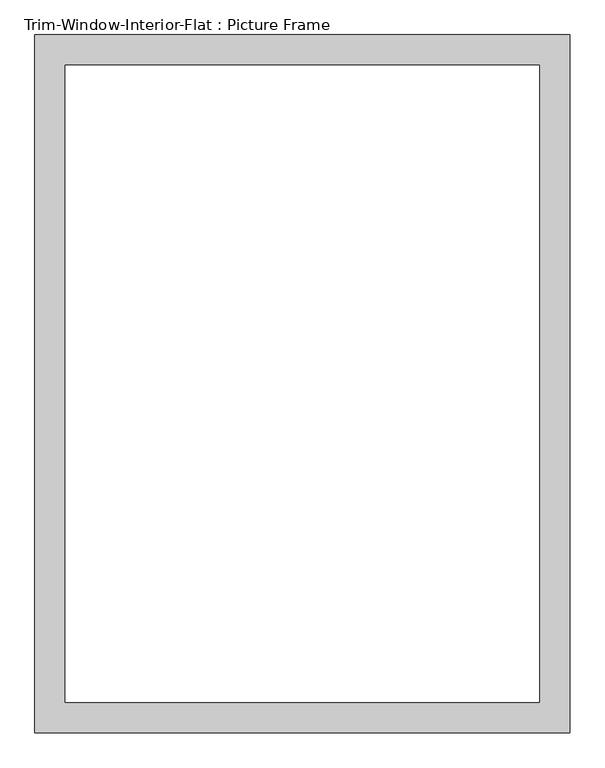
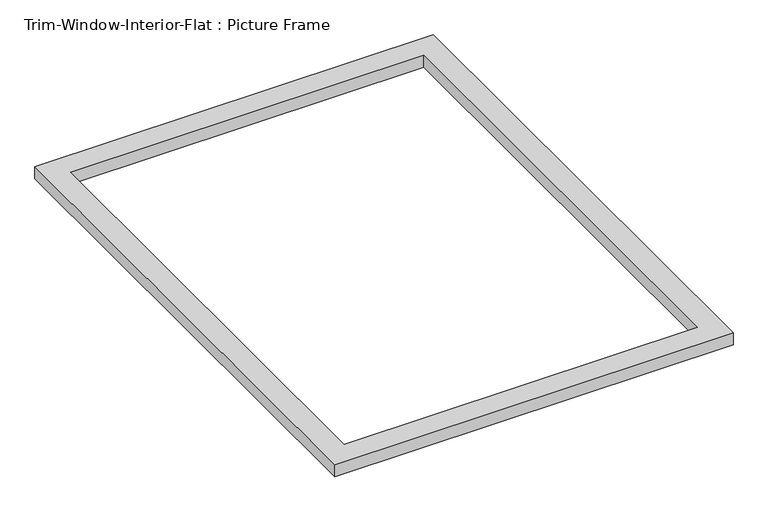
"""IFC4 building model written with IfcOpenShell, lengths in millimetres: proxy geometry, Trim-Window-Interior-Flat : Picture Frame."""

from ifc_helpers import new_model, si_unit, origin, origin_with_axes, place, context, project, spatial, polyline, outline, extrude, source, transform, mapped, element, save


def trim_window_interior_flat_picture_frame_c1dcbb6d(model_context):
    return source(origin(), model_context, "Body", "SweptSolid", [
        extrude(outline(polyline([(501.65, -44.45), (-501.65, -44.45), (-501.65, 1263.65), (501.65, 1263.65), (501.65, -44.45)]), holes=[polyline([(444.5, 12.7), (444.5, 1206.5), (-444.5, 1206.5), (-444.5, 12.7), (444.5, 12.7)])]), origin_with_axes(), (0.0, 0.0, 1.0), 31.75),
    ])


if __name__ == "__main__":
    model = new_model("IFC4")
    model_context = context("Model", 3, world=origin())
    ifc_project = project(units=[si_unit("LENGTHUNIT", "METRE", prefix="MILLI")], contexts=[model_context])
    site = spatial("IfcSite", under=ifc_project)
    building = spatial("IfcBuilding", under=site)
    placement = place(None, origin())
    trim_window_interior_flat_picture_frame_shape = trim_window_interior_flat_picture_frame_c1dcbb6d(model_context)
    element("IfcBuildingElementProxy", 1, Name="Trim-Window-Interior-Flat : Picture Frame", ObjectType="Trim-Window-Interior-Flat : Picture Frame", at=placement, inside=building, context=model_context, shape_type="MappedRepresentation", body=[
        mapped(trim_window_interior_flat_picture_frame_shape, transform((0.0, 0.0, 0.0), x_axis=(1.0, 0.0, 0.0), y_axis=(0.0, 1.0, 0.0), z_axis=(0.0, 0.0, 1.0))),
    ])
    save(model, "model.ifc")

# Revit data of these elements
# Type "Trim-Window-Interior-Flat : Picture Frame"
#   Trim Thickness_Picture Frame = 0' - 1 1/4"
#   Trim Width = 0' - 2 1/4"
#   Trim Thickness_with Sill = 0' - 0 3/4"
#   Sill Thickness = 0' - 1 1/4"
#   Opening Width [instance default] = 2' - 0"
#   Opening Height [instance default] = 3' - 0"
#   Default Elevation = 4' - 0"
#   Sill = no
#   Picture Frame = yes
#   Trim Material [instance default] = none
# Element 1 (IfcBuildingElementProxy, "Trim-Window-Interior-Flat : Picture Frame")
#   Opening Width = 3' - 0"
#   Opening Height = 4' - 0"
#   Trim Material = Wood - Stained
#   Materials on its faces: "Wood - Stained"
# Materials
#   "Wood - Stained": class "Wood", colour RGB 224 178 126, transparency 0, Cost = 0
